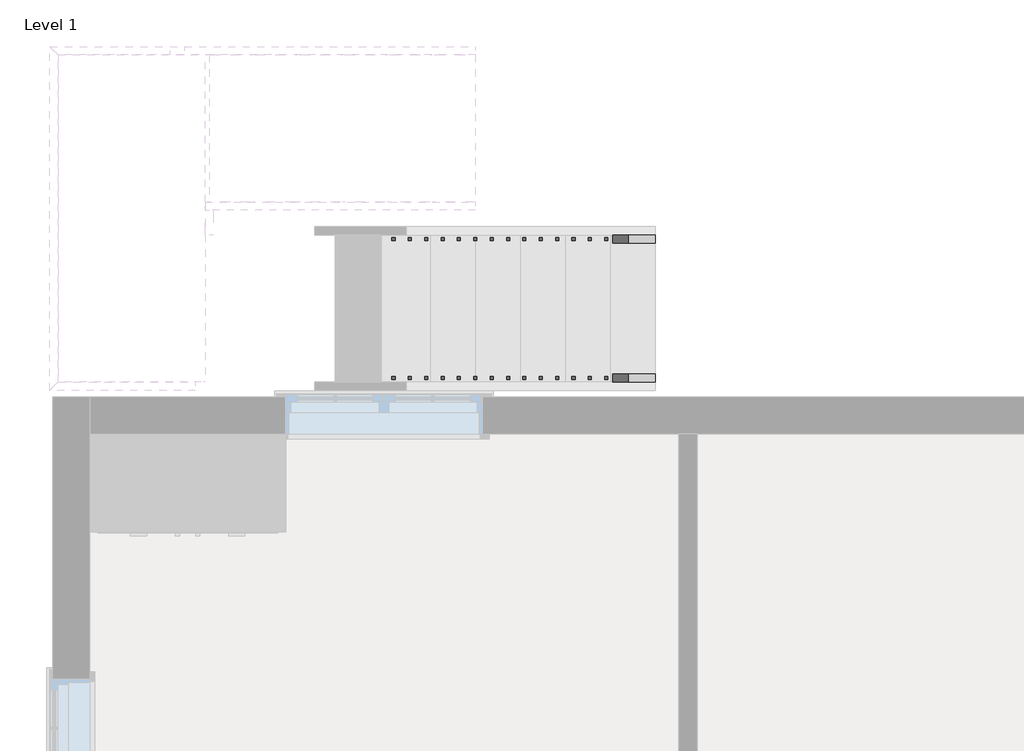
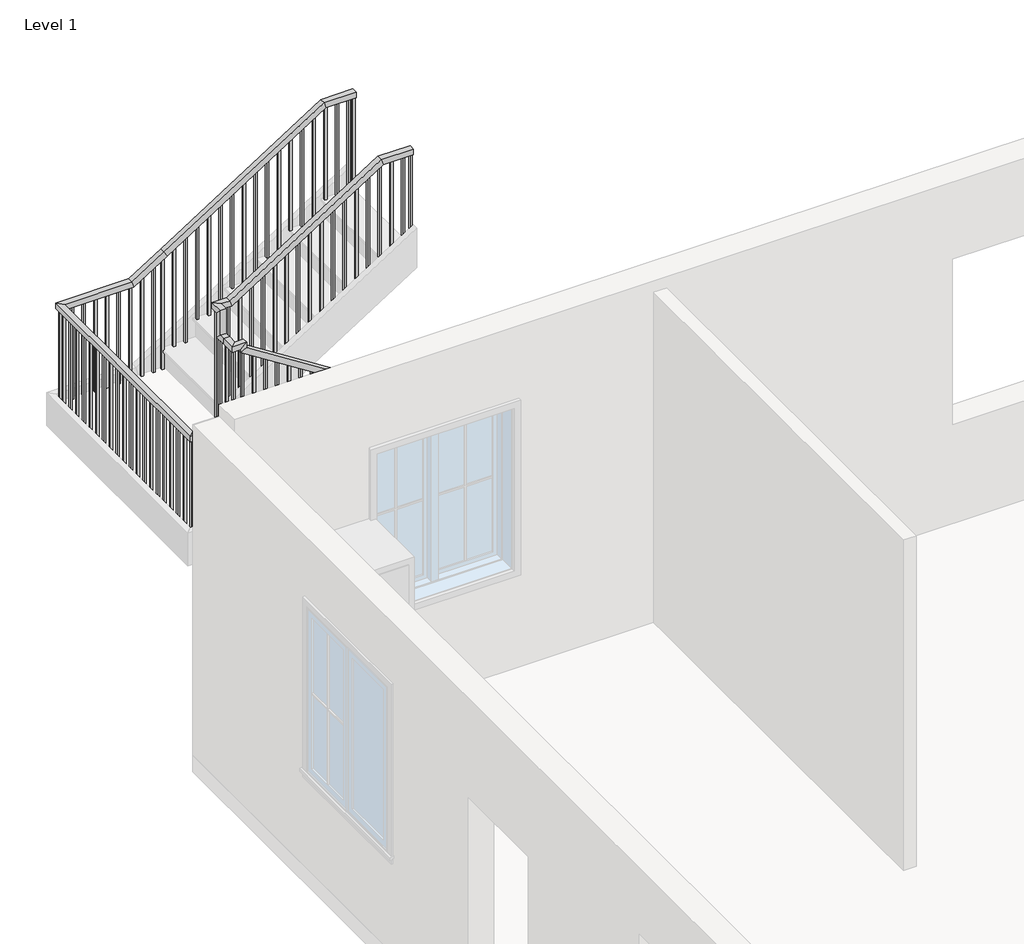
# One storey, part 2 of 3: 2 railings.
"""IFC4 building model written with IfcOpenShell, lengths in millimetres."""

from ifc_helpers import new_model, si_unit, frame, origin, place, context, project, spatial, polyline, outline, extrude, faceted_brep, element, save

model = new_model("IFC4")

# Units and contexts
model_context = context("Model", 3, world=origin())
ifc_project = project(units=[si_unit("LENGTHUNIT", "METRE", prefix="MILLI")], contexts=[model_context])

# Site, building, storey
site = spatial("IfcSite", under=ifc_project)
building = spatial("IfcBuilding", under=site)
storey = spatial("IfcBuildingStorey", under=building, Name="Level 1", Elevation=0.0)

# Railings
placement = place(None, origin())
element("IfcRailing", 1, ObjectType="Handrail - Rectangular", at=placement, inside=storey, context=model_context, shape_type="SolidModel", body=[
    faceted_brep([(13347.9752377, 21750.4384539, 1092.2), (13347.9752377, 21750.4384539, 1031.986276), (13347.9752377, 21801.2384539, 1031.986276), (13347.9752377, 21801.2384539, 1092.2), (10630.1752377, 21750.4384539, 2821.7090909), (10579.3752377, 21750.4384539, 2793.8226396), (10579.3752377, 21801.2384539, 2793.8226396), (10630.1752377, 21801.2384539, 2821.7090909), (10630.1752377, 21750.4384539, 2870.2), (10579.3752377, 21750.4384539, 2819.4), (10579.3752377, 21801.2384539, 2819.4), (10630.1752377, 21801.2384539, 2870.2), (10503.1752377, 21750.4384539, 2870.2), (10503.1752377, 21750.4384539, 2819.4), (10553.9752377, 21801.2384539, 2819.4), (10553.9752377, 21801.2384539, 2870.2), (10503.1752377, 21877.4384539, 2870.2), (10503.1752377, 21877.4384539, 2819.4), (10553.9752377, 21877.4384539, 2819.4), (10553.9752377, 21877.4384539, 2870.2), (10503.1752377, 21930.0919009, 2870.2), (10503.1752377, 21980.8919009, 2819.4), (10553.9752377, 21980.8919009, 2819.4), (10553.9752377, 21930.0919009, 2870.2), (10503.1752377, 21930.0919009, 3096.4909091), (10503.1752377, 21980.8919009, 3045.6909091), (10553.9752377, 21980.8919009, 3045.6909091), (10553.9752377, 21930.0919009, 3096.4909091), (10503.1752377, 22057.0919009, 3096.4909091), (10503.1752377, 22057.0919009, 3045.6909091), (10553.9752377, 22006.2919009, 3045.6909091), (10553.9752377, 22006.2919009, 3096.4909091), (10630.1752377, 22057.0919009, 3096.4909091), (10644.9682326, 22057.0919009, 3045.6909091), (10644.9682326, 22006.2919009, 3045.6909091), (10630.1752377, 22006.2919009, 3096.4909091), (11950.9752377, 22057.0919009, 3937.0), (11965.7682326, 22057.0919009, 3886.2), (11965.7682326, 22006.2919009, 3886.2), (11950.9752377, 22006.2919009, 3937.0), (12230.3752377, 22057.0919009, 3937.0), (12230.3752377, 22006.2919009, 3937.0), (12230.3752377, 22006.2919009, 3886.2), (12230.3752377, 22057.0919009, 3886.2)], [[[0, 1, 2, 3]], [[1, 0, 4, 5]], [[2, 1, 5, 6]], [[3, 2, 6, 7]], [[0, 3, 7, 4]], [[5, 4, 8, 9]], [[6, 5, 9, 10]], [[7, 6, 10, 11]], [[4, 7, 11, 8]], [[9, 8, 12, 13]], [[10, 9, 13, 14]], [[11, 10, 14, 15]], [[8, 11, 15, 12]], [[13, 12, 16, 17]], [[14, 13, 17, 18]], [[15, 14, 18, 19]], [[12, 15, 19, 16]], [[17, 16, 20, 21]], [[18, 17, 21, 22]], [[19, 18, 22, 23]], [[16, 19, 23, 20]], [[21, 20, 24, 25]], [[22, 21, 25, 26]], [[23, 22, 26, 27]], [[20, 23, 27, 24]], [[25, 24, 28, 29]], [[26, 25, 29, 30]], [[27, 26, 30, 31]], [[24, 27, 31, 28]], [[29, 28, 32, 33]], [[30, 29, 33, 34]], [[31, 30, 34, 35]], [[28, 31, 35, 32]], [[33, 32, 36, 37]], [[34, 33, 37, 38]], [[35, 34, 38, 39]], [[32, 35, 39, 36]], [[40, 41, 42, 43]], [[37, 36, 40, 43]], [[38, 37, 43, 42]], [[39, 38, 42, 41]], [[36, 39, 41, 40]]]),
    extrude(outline(polyline([(12144.6502377, 22022.1669009), (12144.6502377, 22041.2169009), (12163.7002377, 22041.2169009), (12163.7002377, 22022.1669009), (12144.6502377, 22022.1669009)])), frame((0.0, 0.0, 3022.6), z_axis=(0.0, 0.0, 1.0), x_axis=(1.0, 0.0, 0.0)), (0.0, 0.0, 1.0), 863.6),
    extrude(outline(polyline([(12043.0502377, 22022.1669009), (12043.0502377, 22041.2169009), (12062.1002377, 22041.2169009), (12062.1002377, 22022.1669009), (12043.0502377, 22022.1669009)])), frame((0.0, 0.0, 3022.6), z_axis=(0.0, 0.0, 1.0), x_axis=(1.0, 0.0, 0.0)), (0.0, 0.0, 1.0), 863.6),
    extrude(outline(polyline([(3882.8476396, 11960.5002377), (3870.7249123, 11941.4502377), (3022.6, 11941.4502377), (3022.6, 11960.5002377), (3882.8476396, 11960.5002377)])), frame((0.0, 22022.1669009, 0.0), z_axis=(0.0, 1.0, 0.0), x_axis=(0.0, 0.0, 1.0)), (0.0, 0.0, 1.0), 19.05),
    extrude(outline(polyline([(3818.1930941, 11858.9002377), (3806.0703669, 11839.8502377), (2844.8, 11839.8502377), (2844.8, 11858.9002377), (3818.1930941, 11858.9002377)])), frame((0.0, 22022.1669009, 0.0), z_axis=(0.0, 1.0, 0.0), x_axis=(0.0, 0.0, 1.0)), (0.0, 0.0, 1.0), 19.05),
    extrude(outline(polyline([(3753.5385487, 11757.3002377), (3741.4158214, 11738.2502377), (2844.8, 11738.2502377), (2844.8, 11757.3002377), (3753.5385487, 11757.3002377)])), frame((0.0, 22022.1669009, 0.0), z_axis=(0.0, 1.0, 0.0), x_axis=(0.0, 0.0, 1.0)), (0.0, 0.0, 1.0), 19.05),
    extrude(outline(polyline([(3688.8840032, 11655.7002377), (3676.761276, 11636.6502377), (2667.0, 11636.6502377), (2667.0, 11655.7002377), (3688.8840032, 11655.7002377)])), frame((0.0, 22022.1669009, 0.0), z_axis=(0.0, 1.0, 0.0), x_axis=(0.0, 0.0, 1.0)), (0.0, 0.0, 1.0), 19.05),
    extrude(outline(polyline([(3624.2294578, 11554.1002377), (3612.1067305, 11535.0502377), (2667.0, 11535.0502377), (2667.0, 11554.1002377), (3624.2294578, 11554.1002377)])), frame((0.0, 22022.1669009, 0.0), z_axis=(0.0, 1.0, 0.0), x_axis=(0.0, 0.0, 1.0)), (0.0, 0.0, 1.0), 19.05),
    extrude(outline(polyline([(3559.5749123, 11452.5002377), (3547.4521851, 11433.4502377), (2667.0, 11433.4502377), (2667.0, 11452.5002377), (3559.5749123, 11452.5002377)])), frame((0.0, 22022.1669009, 0.0), z_axis=(0.0, 1.0, 0.0), x_axis=(0.0, 0.0, 1.0)), (0.0, 0.0, 1.0), 19.05),
    extrude(outline(polyline([(3494.9203669, 11350.9002377), (3482.7976396, 11331.8502377), (2489.2, 11331.8502377), (2489.2, 11350.9002377), (3494.9203669, 11350.9002377)])), frame((0.0, 22022.1669009, 0.0), z_axis=(0.0, 1.0, 0.0), x_axis=(0.0, 0.0, 1.0)), (0.0, 0.0, 1.0), 19.05),
    extrude(outline(polyline([(3430.2658214, 11249.3002377), (3418.1430941, 11230.2502377), (2489.2, 11230.2502377), (2489.2, 11249.3002377), (3430.2658214, 11249.3002377)])), frame((0.0, 22022.1669009, 0.0), z_axis=(0.0, 1.0, 0.0), x_axis=(0.0, 0.0, 1.0)), (0.0, 0.0, 1.0), 19.05),
    extrude(outline(polyline([(3365.611276, 11147.7002377), (3353.4885487, 11128.6502377), (2489.2, 11128.6502377), (2489.2, 11147.7002377), (3365.611276, 11147.7002377)])), frame((0.0, 22022.1669009, 0.0), z_axis=(0.0, 1.0, 0.0), x_axis=(0.0, 0.0, 1.0)), (0.0, 0.0, 1.0), 19.05),
    extrude(outline(polyline([(3300.9567305, 11046.1002377), (3288.8340032, 11027.0502377), (2311.4, 11027.0502377), (2311.4, 11046.1002377), (3300.9567305, 11046.1002377)])), frame((0.0, 22022.1669009, 0.0), z_axis=(0.0, 1.0, 0.0), x_axis=(0.0, 0.0, 1.0)), (0.0, 0.0, 1.0), 19.05),
    extrude(outline(polyline([(3236.3021851, 10944.5002377), (3224.1794578, 10925.4502377), (2311.4, 10925.4502377), (2311.4, 10944.5002377), (3236.3021851, 10944.5002377)])), frame((0.0, 22022.1669009, 0.0), z_axis=(0.0, 1.0, 0.0), x_axis=(0.0, 0.0, 1.0)), (0.0, 0.0, 1.0), 19.05),
    extrude(outline(polyline([(3171.6476396, 10842.9002377), (3159.5249123, 10823.8502377), (2311.4, 10823.8502377), (2311.4, 10842.9002377), (3171.6476396, 10842.9002377)])), frame((0.0, 22022.1669009, 0.0), z_axis=(0.0, 1.0, 0.0), x_axis=(0.0, 0.0, 1.0)), (0.0, 0.0, 1.0), 19.05),
    extrude(outline(polyline([(3106.9930941, 10741.3002377), (3094.8703669, 10722.2502377), (2133.6, 10722.2502377), (2133.6, 10741.3002377), (3106.9930941, 10741.3002377)])), frame((0.0, 22022.1669009, 0.0), z_axis=(0.0, 1.0, 0.0), x_axis=(0.0, 0.0, 1.0)), (0.0, 0.0, 1.0), 19.05),
    extrude(outline(polyline([(3042.3385487, 10639.7002377), (3030.2158214, 10620.6502377), (2133.6, 10620.6502377), (2133.6, 10639.7002377), (3042.3385487, 10639.7002377)])), frame((0.0, 22022.1669009, 0.0), z_axis=(0.0, 1.0, 0.0), x_axis=(0.0, 0.0, 1.0)), (0.0, 0.0, 1.0), 19.05),
    extrude(outline(polyline([(10538.1002377, 21969.5134539), (10519.0502377, 21969.5134539), (10519.0502377, 21988.5634539), (10538.1002377, 21988.5634539), (10538.1002377, 21969.5134539)])), frame((0.0, 0.0, 1955.8), z_axis=(0.0, 0.0, 1.0), x_axis=(1.0, 0.0, 0.0)), (0.0, 0.0, 1.0), 1089.8909091),
    extrude(outline(polyline([(10538.1002377, 21867.9134539), (10519.0502377, 21867.9134539), (10519.0502377, 21886.9634539), (10538.1002377, 21886.9634539), (10538.1002377, 21867.9134539)])), frame((0.0, 0.0, 1955.8), z_axis=(0.0, 0.0, 1.0), x_axis=(1.0, 0.0, 0.0)), (0.0, 0.0, 1.0), 863.6),
    extrude(outline(polyline([(10614.3002377, 21785.3634539), (10614.3002377, 21766.3134539), (10595.2502377, 21766.3134539), (10595.2502377, 21785.3634539), (10614.3002377, 21785.3634539)])), frame((0.0, 0.0, 1778.0), z_axis=(0.0, 0.0, 1.0), x_axis=(1.0, 0.0, 0.0)), (0.0, 0.0, 1.0), 1041.4),
    extrude(outline(polyline([(2706.9430941, 10715.9002377), (2719.0658214, 10696.8502377), (1778.0, 10696.8502377), (1778.0, 10715.9002377), (2706.9430941, 10715.9002377)])), frame((0.0, 21766.3134539, 0.0), z_axis=(0.0, 1.0, 0.0), x_axis=(0.0, 0.0, 1.0)), (0.0, 0.0, 1.0), 19.05),
    extrude(outline(polyline([(2642.2885487, 10817.5002377), (2654.411276, 10798.4502377), (1778.0, 10798.4502377), (1778.0, 10817.5002377), (2642.2885487, 10817.5002377)])), frame((0.0, 21766.3134539, 0.0), z_axis=(0.0, 1.0, 0.0), x_axis=(0.0, 0.0, 1.0)), (0.0, 0.0, 1.0), 19.05),
    extrude(outline(polyline([(2577.6340032, 10919.1002377), (2589.7567305, 10900.0502377), (1600.2, 10900.0502377), (1600.2, 10919.1002377), (2577.6340032, 10919.1002377)])), frame((0.0, 21766.3134539, 0.0), z_axis=(0.0, 1.0, 0.0), x_axis=(0.0, 0.0, 1.0)), (0.0, 0.0, 1.0), 19.05),
    extrude(outline(polyline([(2512.9794578, 11020.7002377), (2525.1021851, 11001.6502377), (1600.2, 11001.6502377), (1600.2, 11020.7002377), (2512.9794578, 11020.7002377)])), frame((0.0, 21766.3134539, 0.0), z_axis=(0.0, 1.0, 0.0), x_axis=(0.0, 0.0, 1.0)), (0.0, 0.0, 1.0), 19.05),
    extrude(outline(polyline([(2448.3249123, 11122.3002377), (2460.4476396, 11103.2502377), (1600.2, 11103.2502377), (1600.2, 11122.3002377), (2448.3249123, 11122.3002377)])), frame((0.0, 21766.3134539, 0.0), z_axis=(0.0, 1.0, 0.0), x_axis=(0.0, 0.0, 1.0)), (0.0, 0.0, 1.0), 19.05),
    extrude(outline(polyline([(2383.6703669, 11223.9002377), (2395.7930941, 11204.8502377), (1422.4, 11204.8502377), (1422.4, 11223.9002377), (2383.6703669, 11223.9002377)])), frame((0.0, 21766.3134539, 0.0), z_axis=(0.0, 1.0, 0.0), x_axis=(0.0, 0.0, 1.0)), (0.0, 0.0, 1.0), 19.05),
    extrude(outline(polyline([(2319.0158214, 11325.5002377), (2331.1385487, 11306.4502377), (1422.4, 11306.4502377), (1422.4, 11325.5002377), (2319.0158214, 11325.5002377)])), frame((0.0, 21766.3134539, 0.0), z_axis=(0.0, 1.0, 0.0), x_axis=(0.0, 0.0, 1.0)), (0.0, 0.0, 1.0), 19.05),
    extrude(outline(polyline([(2254.361276, 11427.1002377), (2266.4840032, 11408.0502377), (1244.6, 11408.0502377), (1244.6, 11427.1002377), (2254.361276, 11427.1002377)])), frame((0.0, 21766.3134539, 0.0), z_axis=(0.0, 1.0, 0.0), x_axis=(0.0, 0.0, 1.0)), (0.0, 0.0, 1.0), 19.05),
    extrude(outline(polyline([(2189.7067305, 11528.7002377), (2201.8294578, 11509.6502377), (1244.6, 11509.6502377), (1244.6, 11528.7002377), (2189.7067305, 11528.7002377)])), frame((0.0, 21766.3134539, 0.0), z_axis=(0.0, 1.0, 0.0), x_axis=(0.0, 0.0, 1.0)), (0.0, 0.0, 1.0), 19.05),
    extrude(outline(polyline([(2125.0521851, 11630.3002377), (2137.1749123, 11611.2502377), (1244.6, 11611.2502377), (1244.6, 11630.3002377), (2125.0521851, 11630.3002377)])), frame((0.0, 21766.3134539, 0.0), z_axis=(0.0, 1.0, 0.0), x_axis=(0.0, 0.0, 1.0)), (0.0, 0.0, 1.0), 19.05),
    extrude(outline(polyline([(2060.3976396, 11731.9002377), (2072.5203669, 11712.8502377), (1066.8, 11712.8502377), (1066.8, 11731.9002377), (2060.3976396, 11731.9002377)])), frame((0.0, 21766.3134539, 0.0), z_axis=(0.0, 1.0, 0.0), x_axis=(0.0, 0.0, 1.0)), (0.0, 0.0, 1.0), 19.05),
    extrude(outline(polyline([(1995.7430941, 11833.5002377), (2007.8658214, 11814.4502377), (1066.8, 11814.4502377), (1066.8, 11833.5002377), (1995.7430941, 11833.5002377)])), frame((0.0, 21766.3134539, 0.0), z_axis=(0.0, 1.0, 0.0), x_axis=(0.0, 0.0, 1.0)), (0.0, 0.0, 1.0), 19.05),
    extrude(outline(polyline([(1931.0885487, 11935.1002377), (1943.211276, 11916.0502377), (1066.8, 11916.0502377), (1066.8, 11935.1002377), (1931.0885487, 11935.1002377)])), frame((0.0, 21766.3134539, 0.0), z_axis=(0.0, 1.0, 0.0), x_axis=(0.0, 0.0, 1.0)), (0.0, 0.0, 1.0), 19.05),
    extrude(outline(polyline([(1866.4340032, 12036.7002377), (1878.5567305, 12017.6502377), (889.0, 12017.6502377), (889.0, 12036.7002377), (1866.4340032, 12036.7002377)])), frame((0.0, 21766.3134539, 0.0), z_axis=(0.0, 1.0, 0.0), x_axis=(0.0, 0.0, 1.0)), (0.0, 0.0, 1.0), 19.05),
    extrude(outline(polyline([(1801.7794578, 12138.3002377), (1813.9021851, 12119.2502377), (889.0, 12119.2502377), (889.0, 12138.3002377), (1801.7794578, 12138.3002377)])), frame((0.0, 21766.3134539, 0.0), z_axis=(0.0, 1.0, 0.0), x_axis=(0.0, 0.0, 1.0)), (0.0, 0.0, 1.0), 19.05),
    extrude(outline(polyline([(1737.1249123, 12239.9002377), (1749.2476396, 12220.8502377), (889.0, 12220.8502377), (889.0, 12239.9002377), (1737.1249123, 12239.9002377)])), frame((0.0, 21766.3134539, 0.0), z_axis=(0.0, 1.0, 0.0), x_axis=(0.0, 0.0, 1.0)), (0.0, 0.0, 1.0), 19.05),
    extrude(outline(polyline([(1672.4703669, 12341.5002377), (1684.5930941, 12322.4502377), (711.2, 12322.4502377), (711.2, 12341.5002377), (1672.4703669, 12341.5002377)])), frame((0.0, 21766.3134539, 0.0), z_axis=(0.0, 1.0, 0.0), x_axis=(0.0, 0.0, 1.0)), (0.0, 0.0, 1.0), 19.05),
    extrude(outline(polyline([(1607.8158214, 12443.1002377), (1619.9385487, 12424.0502377), (711.2, 12424.0502377), (711.2, 12443.1002377), (1607.8158214, 12443.1002377)])), frame((0.0, 21766.3134539, 0.0), z_axis=(0.0, 1.0, 0.0), x_axis=(0.0, 0.0, 1.0)), (0.0, 0.0, 1.0), 19.05),
    extrude(outline(polyline([(1543.161276, 12544.7002377), (1555.2840032, 12525.6502377), (533.4, 12525.6502377), (533.4, 12544.7002377), (1543.161276, 12544.7002377)])), frame((0.0, 21766.3134539, 0.0), z_axis=(0.0, 1.0, 0.0), x_axis=(0.0, 0.0, 1.0)), (0.0, 0.0, 1.0), 19.05),
    extrude(outline(polyline([(1478.5067305, 12646.3002377), (1490.6294578, 12627.2502377), (533.4, 12627.2502377), (533.4, 12646.3002377), (1478.5067305, 12646.3002377)])), frame((0.0, 21766.3134539, 0.0), z_axis=(0.0, 1.0, 0.0), x_axis=(0.0, 0.0, 1.0)), (0.0, 0.0, 1.0), 19.05),
    extrude(outline(polyline([(1413.8521851, 12747.9002377), (1425.9749123, 12728.8502377), (533.4, 12728.8502377), (533.4, 12747.9002377), (1413.8521851, 12747.9002377)])), frame((0.0, 21766.3134539, 0.0), z_axis=(0.0, 1.0, 0.0), x_axis=(0.0, 0.0, 1.0)), (0.0, 0.0, 1.0), 19.05),
    extrude(outline(polyline([(1349.1976396, 12849.5002377), (1361.3203669, 12830.4502377), (355.6, 12830.4502377), (355.6, 12849.5002377), (1349.1976396, 12849.5002377)])), frame((0.0, 21766.3134539, 0.0), z_axis=(0.0, 1.0, 0.0), x_axis=(0.0, 0.0, 1.0)), (0.0, 0.0, 1.0), 19.05),
    extrude(outline(polyline([(1284.5430941, 12951.1002377), (1296.6658214, 12932.0502377), (355.6, 12932.0502377), (355.6, 12951.1002377), (1284.5430941, 12951.1002377)])), frame((0.0, 21766.3134539, 0.0), z_axis=(0.0, 1.0, 0.0), x_axis=(0.0, 0.0, 1.0)), (0.0, 0.0, 1.0), 19.05),
    extrude(outline(polyline([(1219.8885487, 13052.7002377), (1232.011276, 13033.6502377), (355.6, 13033.6502377), (355.6, 13052.7002377), (1219.8885487, 13052.7002377)])), frame((0.0, 21766.3134539, 0.0), z_axis=(0.0, 1.0, 0.0), x_axis=(0.0, 0.0, 1.0)), (0.0, 0.0, 1.0), 19.05),
    extrude(outline(polyline([(1155.2340032, 13154.3002377), (1167.3567305, 13135.2502377), (177.8, 13135.2502377), (177.8, 13154.3002377), (1155.2340032, 13154.3002377)])), frame((0.0, 21766.3134539, 0.0), z_axis=(0.0, 1.0, 0.0), x_axis=(0.0, 0.0, 1.0)), (0.0, 0.0, 1.0), 19.05),
    extrude(outline(polyline([(1090.5794578, 13255.9002377), (1102.7021851, 13236.8502377), (177.8, 13236.8502377), (177.8, 13255.9002377), (1090.5794578, 13255.9002377)])), frame((0.0, 21766.3134539, 0.0), z_axis=(0.0, 1.0, 0.0), x_axis=(0.0, 0.0, 1.0)), (0.0, 0.0, 1.0), 19.05),
    extrude(outline(polyline([(10538.1002377, 22022.1669009), (10519.0502377, 22022.1669009), (10519.0502377, 22041.2169009), (10538.1002377, 22041.2169009), (10538.1002377, 22022.1669009)])), frame((0.0, 0.0, 1955.8), z_axis=(0.0, 0.0, 1.0), x_axis=(1.0, 0.0, 0.0)), (0.0, 0.0, 1.0), 1089.8909091),
    extrude(outline(polyline([(10538.1002377, 21785.3634539), (10538.1002377, 21766.3134539), (10519.0502377, 21766.3134539), (10519.0502377, 21785.3634539), (10538.1002377, 21785.3634539)])), frame((0.0, 0.0, 1955.8), z_axis=(0.0, 0.0, 1.0), x_axis=(1.0, 0.0, 0.0)), (0.0, 0.0, 1.0), 863.6),
    extrude(outline(polyline([(12211.3252377, 22022.1669009), (12211.3252377, 22041.2169009), (12230.3752377, 22041.2169009), (12230.3752377, 22022.1669009), (12211.3252377, 22022.1669009)])), frame((0.0, 0.0, 3022.6), z_axis=(0.0, 0.0, 1.0), x_axis=(1.0, 0.0, 0.0)), (0.0, 0.0, 1.0), 863.6),
    extrude(outline(polyline([(1031.986276, 13347.9752377), (1044.1090032, 13328.9252377), (177.8, 13328.9252377), (177.8, 13347.9752377), (1031.986276, 13347.9752377)])), frame((0.0, 21766.3134539, 0.0), z_axis=(0.0, 1.0, 0.0), x_axis=(0.0, 0.0, 1.0)), (0.0, 0.0, 1.0), 19.05),
])
element("IfcRailing", 2, ObjectType="Handrail - Rectangular", at=placement, inside=storey, context=model_context, shape_type="SolidModel", body=[
    faceted_brep([(13347.9752377, 20886.8384539, 1092.2), (13347.9752377, 20886.8384539, 1031.986276), (13347.9752377, 20937.6384539, 1031.986276), (13347.9752377, 20937.6384539, 1092.2), (10553.9752377, 20886.8384539, 2870.2), (10539.1822428, 20886.8384539, 2819.4), (10539.1822428, 20937.6384539, 2819.4), (10553.9752377, 20937.6384539, 2870.2), (9639.5752377, 20886.8384539, 2870.2), (9639.5752377, 20886.8384539, 2819.4), (9690.3752377, 20937.6384539, 2819.4), (9690.3752377, 20937.6384539, 2870.2), (9639.5752377, 22920.6919009, 2870.2), (9639.5752377, 22920.6919009, 2819.4), (9690.3752377, 22869.8919009, 2819.4), (9690.3752377, 22869.8919009, 2870.2), (10274.5752377, 22920.6919009, 2870.2), (10289.3682326, 22920.6919009, 2819.4), (10289.3682326, 22869.8919009, 2819.4), (10274.5752377, 22869.8919009, 2870.2), (10553.9752377, 22920.6919009, 3048.0), (10581.2485127, 22920.6919009, 3005.1419964), (10581.2485127, 22869.8919009, 3005.1419964), (10553.9752377, 22869.8919009, 3048.0), (11950.9752377, 22920.6919009, 3937.0), (11965.7682326, 22920.6919009, 3886.2), (11965.7682326, 22869.8919009, 3886.2), (11950.9752377, 22869.8919009, 3937.0), (12230.3752377, 22920.6919009, 3937.0), (12230.3752377, 22869.8919009, 3937.0), (12230.3752377, 22869.8919009, 3886.2), (12230.3752377, 22920.6919009, 3886.2)], [[[0, 1, 2, 3]], [[1, 0, 4, 5]], [[2, 1, 5, 6]], [[3, 2, 6, 7]], [[0, 3, 7, 4]], [[5, 4, 8, 9]], [[6, 5, 9, 10]], [[7, 6, 10, 11]], [[4, 7, 11, 8]], [[9, 8, 12, 13]], [[10, 9, 13, 14]], [[11, 10, 14, 15]], [[8, 11, 15, 12]], [[13, 12, 16, 17]], [[14, 13, 17, 18]], [[15, 14, 18, 19]], [[12, 15, 19, 16]], [[17, 16, 20, 21]], [[18, 17, 21, 22]], [[19, 18, 22, 23]], [[16, 19, 23, 20]], [[21, 20, 24, 25]], [[22, 21, 25, 26]], [[23, 22, 26, 27]], [[20, 23, 27, 24]], [[28, 29, 30, 31]], [[25, 24, 28, 31]], [[26, 25, 31, 30]], [[27, 26, 30, 29]], [[24, 27, 29, 28]]]),
    extrude(outline(polyline([(12170.0502377, 22904.8169009), (12189.1002377, 22904.8169009), (12189.1002377, 22885.7669009), (12170.0502377, 22885.7669009), (12170.0502377, 22904.8169009)])), frame((0.0, 0.0, 3022.6), z_axis=(0.0, 0.0, 1.0), x_axis=(1.0, 0.0, 0.0)), (0.0, 0.0, 1.0), 863.6),
    extrude(outline(polyline([(12068.4502377, 22904.8169009), (12087.5002377, 22904.8169009), (12087.5002377, 22885.7669009), (12068.4502377, 22885.7669009), (12068.4502377, 22904.8169009)])), frame((0.0, 0.0, 3022.6), z_axis=(0.0, 0.0, 1.0), x_axis=(1.0, 0.0, 0.0)), (0.0, 0.0, 1.0), 863.6),
    extrude(outline(polyline([(11966.8502377, 22904.8169009), (11985.9002377, 22904.8169009), (11985.9002377, 22885.7669009), (11966.8502377, 22885.7669009), (11966.8502377, 22904.8169009)])), frame((0.0, 0.0, 3022.6), z_axis=(0.0, 0.0, 1.0), x_axis=(1.0, 0.0, 0.0)), (0.0, 0.0, 1.0), 863.6),
    extrude(outline(polyline([(3822.2340032, 11865.2502377), (2844.8, 11865.2502377), (2844.8, 11884.3002377), (3834.3567305, 11884.3002377), (3822.2340032, 11865.2502377)])), frame((0.0, 22885.7669009, 0.0), z_axis=(0.0, 1.0, 0.0), x_axis=(0.0, 0.0, 1.0)), (0.0, 0.0, 1.0), 19.05),
    extrude(outline(polyline([(3757.5794578, 11763.6502377), (2844.8, 11763.6502377), (2844.8, 11782.7002377), (3769.7021851, 11782.7002377), (3757.5794578, 11763.6502377)])), frame((0.0, 22885.7669009, 0.0), z_axis=(0.0, 1.0, 0.0), x_axis=(0.0, 0.0, 1.0)), (0.0, 0.0, 1.0), 19.05),
    extrude(outline(polyline([(3692.9249123, 11662.0502377), (2844.8, 11662.0502377), (2844.8, 11681.1002377), (3705.0476396, 11681.1002377), (3692.9249123, 11662.0502377)])), frame((0.0, 22885.7669009, 0.0), z_axis=(0.0, 1.0, 0.0), x_axis=(0.0, 0.0, 1.0)), (0.0, 0.0, 1.0), 19.05),
    extrude(outline(polyline([(3628.2703669, 11560.4502377), (2667.0, 11560.4502377), (2667.0, 11579.5002377), (3640.3930941, 11579.5002377), (3628.2703669, 11560.4502377)])), frame((0.0, 22885.7669009, 0.0), z_axis=(0.0, 1.0, 0.0), x_axis=(0.0, 0.0, 1.0)), (0.0, 0.0, 1.0), 19.05),
    extrude(outline(polyline([(3563.6158214, 11458.8502377), (2667.0, 11458.8502377), (2667.0, 11477.9002377), (3575.7385487, 11477.9002377), (3563.6158214, 11458.8502377)])), frame((0.0, 22885.7669009, 0.0), z_axis=(0.0, 1.0, 0.0), x_axis=(0.0, 0.0, 1.0)), (0.0, 0.0, 1.0), 19.05),
    extrude(outline(polyline([(3498.961276, 11357.2502377), (2489.2, 11357.2502377), (2489.2, 11376.3002377), (3511.0840032, 11376.3002377), (3498.961276, 11357.2502377)])), frame((0.0, 22885.7669009, 0.0), z_axis=(0.0, 1.0, 0.0), x_axis=(0.0, 0.0, 1.0)), (0.0, 0.0, 1.0), 19.05),
    extrude(outline(polyline([(3434.3067305, 11255.6502377), (2489.2, 11255.6502377), (2489.2, 11274.7002377), (3446.4294578, 11274.7002377), (3434.3067305, 11255.6502377)])), frame((0.0, 22885.7669009, 0.0), z_axis=(0.0, 1.0, 0.0), x_axis=(0.0, 0.0, 1.0)), (0.0, 0.0, 1.0), 19.05),
    extrude(outline(polyline([(3369.6521851, 11154.0502377), (2489.2, 11154.0502377), (2489.2, 11173.1002377), (3381.7749123, 11173.1002377), (3369.6521851, 11154.0502377)])), frame((0.0, 22885.7669009, 0.0), z_axis=(0.0, 1.0, 0.0), x_axis=(0.0, 0.0, 1.0)), (0.0, 0.0, 1.0), 19.05),
    extrude(outline(polyline([(3304.9976396, 11052.4502377), (2311.4, 11052.4502377), (2311.4, 11071.5002377), (3317.1203669, 11071.5002377), (3304.9976396, 11052.4502377)])), frame((0.0, 22885.7669009, 0.0), z_axis=(0.0, 1.0, 0.0), x_axis=(0.0, 0.0, 1.0)), (0.0, 0.0, 1.0), 19.05),
    extrude(outline(polyline([(3240.3430941, 10950.8502377), (2311.4, 10950.8502377), (2311.4, 10969.9002377), (3252.4658214, 10969.9002377), (3240.3430941, 10950.8502377)])), frame((0.0, 22885.7669009, 0.0), z_axis=(0.0, 1.0, 0.0), x_axis=(0.0, 0.0, 1.0)), (0.0, 0.0, 1.0), 19.05),
    extrude(outline(polyline([(3175.6885487, 10849.2502377), (2311.4, 10849.2502377), (2311.4, 10868.3002377), (3187.811276, 10868.3002377), (3175.6885487, 10849.2502377)])), frame((0.0, 22885.7669009, 0.0), z_axis=(0.0, 1.0, 0.0), x_axis=(0.0, 0.0, 1.0)), (0.0, 0.0, 1.0), 19.05),
    extrude(outline(polyline([(3111.0340032, 10747.6502377), (2133.6, 10747.6502377), (2133.6, 10766.7002377), (3123.1567305, 10766.7002377), (3111.0340032, 10747.6502377)])), frame((0.0, 22885.7669009, 0.0), z_axis=(0.0, 1.0, 0.0), x_axis=(0.0, 0.0, 1.0)), (0.0, 0.0, 1.0), 19.05),
    extrude(outline(polyline([(3046.3794578, 10646.0502377), (2133.6, 10646.0502377), (2133.6, 10665.1002377), (3058.5021851, 10665.1002377), (3046.3794578, 10646.0502377)])), frame((0.0, 22885.7669009, 0.0), z_axis=(0.0, 1.0, 0.0), x_axis=(0.0, 0.0, 1.0)), (0.0, 0.0, 1.0), 19.05),
    extrude(outline(polyline([(2933.2340032, 10468.2502377), (1955.8, 10468.2502377), (1955.8, 10487.3002377), (2945.3567305, 10487.3002377), (2933.2340032, 10468.2502377)])), frame((0.0, 22885.7669009, 0.0), z_axis=(0.0, 1.0, 0.0), x_axis=(0.0, 0.0, 1.0)), (0.0, 0.0, 1.0), 19.05),
    extrude(outline(polyline([(2868.5794578, 10366.6502377), (1955.8, 10366.6502377), (1955.8, 10385.7002377), (2880.7021851, 10385.7002377), (2868.5794578, 10366.6502377)])), frame((0.0, 22885.7669009, 0.0), z_axis=(0.0, 1.0, 0.0), x_axis=(0.0, 0.0, 1.0)), (0.0, 0.0, 1.0), 19.05),
    extrude(outline(polyline([(10265.0502377, 22904.8169009), (10284.1002377, 22904.8169009), (10284.1002377, 22885.7669009), (10265.0502377, 22885.7669009), (10265.0502377, 22904.8169009)])), frame((0.0, 0.0, 1955.8), z_axis=(0.0, 0.0, 1.0), x_axis=(1.0, 0.0, 0.0)), (0.0, 0.0, 1.0), 863.6),
    extrude(outline(polyline([(10163.4502377, 22904.8169009), (10182.5002377, 22904.8169009), (10182.5002377, 22885.7669009), (10163.4502377, 22885.7669009), (10163.4502377, 22904.8169009)])), frame((0.0, 0.0, 1955.8), z_axis=(0.0, 0.0, 1.0), x_axis=(1.0, 0.0, 0.0)), (0.0, 0.0, 1.0), 863.6),
    extrude(outline(polyline([(10061.8502377, 22904.8169009), (10080.9002377, 22904.8169009), (10080.9002377, 22885.7669009), (10061.8502377, 22885.7669009), (10061.8502377, 22904.8169009)])), frame((0.0, 0.0, 1955.8), z_axis=(0.0, 0.0, 1.0), x_axis=(1.0, 0.0, 0.0)), (0.0, 0.0, 1.0), 863.6),
    extrude(outline(polyline([(9960.2502377, 22904.8169009), (9979.3002377, 22904.8169009), (9979.3002377, 22885.7669009), (9960.2502377, 22885.7669009), (9960.2502377, 22904.8169009)])), frame((0.0, 0.0, 1955.8), z_axis=(0.0, 0.0, 1.0), x_axis=(1.0, 0.0, 0.0)), (0.0, 0.0, 1.0), 863.6),
    extrude(outline(polyline([(9858.6502377, 22904.8169009), (9877.7002377, 22904.8169009), (9877.7002377, 22885.7669009), (9858.6502377, 22885.7669009), (9858.6502377, 22904.8169009)])), frame((0.0, 0.0, 1955.8), z_axis=(0.0, 0.0, 1.0), x_axis=(1.0, 0.0, 0.0)), (0.0, 0.0, 1.0), 863.6),
    extrude(outline(polyline([(9757.0502377, 22904.8169009), (9776.1002377, 22904.8169009), (9776.1002377, 22885.7669009), (9757.0502377, 22885.7669009), (9757.0502377, 22904.8169009)])), frame((0.0, 0.0, 1955.8), z_axis=(0.0, 0.0, 1.0), x_axis=(1.0, 0.0, 0.0)), (0.0, 0.0, 1.0), 863.6),
    extrude(outline(polyline([(9655.4502377, 22833.1134539), (9655.4502377, 22852.1634539), (9674.5002377, 22852.1634539), (9674.5002377, 22833.1134539), (9655.4502377, 22833.1134539)])), frame((0.0, 0.0, 1955.8), z_axis=(0.0, 0.0, 1.0), x_axis=(1.0, 0.0, 0.0)), (0.0, 0.0, 1.0), 863.6),
    extrude(outline(polyline([(9655.4502377, 22731.5134539), (9655.4502377, 22750.5634539), (9674.5002377, 22750.5634539), (9674.5002377, 22731.5134539), (9655.4502377, 22731.5134539)])), frame((0.0, 0.0, 1955.8), z_axis=(0.0, 0.0, 1.0), x_axis=(1.0, 0.0, 0.0)), (0.0, 0.0, 1.0), 863.6),
    extrude(outline(polyline([(9655.4502377, 22629.9134539), (9655.4502377, 22648.9634539), (9674.5002377, 22648.9634539), (9674.5002377, 22629.9134539), (9655.4502377, 22629.9134539)])), frame((0.0, 0.0, 1955.8), z_axis=(0.0, 0.0, 1.0), x_axis=(1.0, 0.0, 0.0)), (0.0, 0.0, 1.0), 863.6),
    extrude(outline(polyline([(9655.4502377, 22528.3134539), (9655.4502377, 22547.3634539), (9674.5002377, 22547.3634539), (9674.5002377, 22528.3134539), (9655.4502377, 22528.3134539)])), frame((0.0, 0.0, 1955.8), z_axis=(0.0, 0.0, 1.0), x_axis=(1.0, 0.0, 0.0)), (0.0, 0.0, 1.0), 863.6),
    extrude(outline(polyline([(9655.4502377, 22426.7134539), (9655.4502377, 22445.7634539), (9674.5002377, 22445.7634539), (9674.5002377, 22426.7134539), (9655.4502377, 22426.7134539)])), frame((0.0, 0.0, 1955.8), z_axis=(0.0, 0.0, 1.0), x_axis=(1.0, 0.0, 0.0)), (0.0, 0.0, 1.0), 863.6),
    extrude(outline(polyline([(9655.4502377, 22325.1134539), (9655.4502377, 22344.1634539), (9674.5002377, 22344.1634539), (9674.5002377, 22325.1134539), (9655.4502377, 22325.1134539)])), frame((0.0, 0.0, 1955.8), z_axis=(0.0, 0.0, 1.0), x_axis=(1.0, 0.0, 0.0)), (0.0, 0.0, 1.0), 863.6),
    extrude(outline(polyline([(9655.4502377, 22223.5134539), (9655.4502377, 22242.5634539), (9674.5002377, 22242.5634539), (9674.5002377, 22223.5134539), (9655.4502377, 22223.5134539)])), frame((0.0, 0.0, 1955.8), z_axis=(0.0, 0.0, 1.0), x_axis=(1.0, 0.0, 0.0)), (0.0, 0.0, 1.0), 863.6),
    extrude(outline(polyline([(9655.4502377, 22121.9134539), (9655.4502377, 22140.9634539), (9674.5002377, 22140.9634539), (9674.5002377, 22121.9134539), (9655.4502377, 22121.9134539)])), frame((0.0, 0.0, 1955.8), z_axis=(0.0, 0.0, 1.0), x_axis=(1.0, 0.0, 0.0)), (0.0, 0.0, 1.0), 863.6),
    extrude(outline(polyline([(9655.4502377, 22020.3134539), (9655.4502377, 22039.3634539), (9674.5002377, 22039.3634539), (9674.5002377, 22020.3134539), (9655.4502377, 22020.3134539)])), frame((0.0, 0.0, 1955.8), z_axis=(0.0, 0.0, 1.0), x_axis=(1.0, 0.0, 0.0)), (0.0, 0.0, 1.0), 863.6),
    extrude(outline(polyline([(9655.4502377, 21918.7134539), (9655.4502377, 21937.7634539), (9674.5002377, 21937.7634539), (9674.5002377, 21918.7134539), (9655.4502377, 21918.7134539)])), frame((0.0, 0.0, 1955.8), z_axis=(0.0, 0.0, 1.0), x_axis=(1.0, 0.0, 0.0)), (0.0, 0.0, 1.0), 863.6),
    extrude(outline(polyline([(9655.4502377, 21817.1134539), (9655.4502377, 21836.1634539), (9674.5002377, 21836.1634539), (9674.5002377, 21817.1134539), (9655.4502377, 21817.1134539)])), frame((0.0, 0.0, 1955.8), z_axis=(0.0, 0.0, 1.0), x_axis=(1.0, 0.0, 0.0)), (0.0, 0.0, 1.0), 863.6),
    extrude(outline(polyline([(9655.4502377, 21715.5134539), (9655.4502377, 21734.5634539), (9674.5002377, 21734.5634539), (9674.5002377, 21715.5134539), (9655.4502377, 21715.5134539)])), frame((0.0, 0.0, 1955.8), z_axis=(0.0, 0.0, 1.0), x_axis=(1.0, 0.0, 0.0)), (0.0, 0.0, 1.0), 863.6),
    extrude(outline(polyline([(9655.4502377, 21613.9134539), (9655.4502377, 21632.9634539), (9674.5002377, 21632.9634539), (9674.5002377, 21613.9134539), (9655.4502377, 21613.9134539)])), frame((0.0, 0.0, 1955.8), z_axis=(0.0, 0.0, 1.0), x_axis=(1.0, 0.0, 0.0)), (0.0, 0.0, 1.0), 863.6),
    extrude(outline(polyline([(9655.4502377, 21512.3134539), (9655.4502377, 21531.3634539), (9674.5002377, 21531.3634539), (9674.5002377, 21512.3134539), (9655.4502377, 21512.3134539)])), frame((0.0, 0.0, 1955.8), z_axis=(0.0, 0.0, 1.0), x_axis=(1.0, 0.0, 0.0)), (0.0, 0.0, 1.0), 863.6),
    extrude(outline(polyline([(9655.4502377, 21410.7134539), (9655.4502377, 21429.7634539), (9674.5002377, 21429.7634539), (9674.5002377, 21410.7134539), (9655.4502377, 21410.7134539)])), frame((0.0, 0.0, 1955.8), z_axis=(0.0, 0.0, 1.0), x_axis=(1.0, 0.0, 0.0)), (0.0, 0.0, 1.0), 863.6),
    extrude(outline(polyline([(9655.4502377, 21309.1134539), (9655.4502377, 21328.1634539), (9674.5002377, 21328.1634539), (9674.5002377, 21309.1134539), (9655.4502377, 21309.1134539)])), frame((0.0, 0.0, 1955.8), z_axis=(0.0, 0.0, 1.0), x_axis=(1.0, 0.0, 0.0)), (0.0, 0.0, 1.0), 863.6),
    extrude(outline(polyline([(9655.4502377, 21207.5134539), (9655.4502377, 21226.5634539), (9674.5002377, 21226.5634539), (9674.5002377, 21207.5134539), (9655.4502377, 21207.5134539)])), frame((0.0, 0.0, 1955.8), z_axis=(0.0, 0.0, 1.0), x_axis=(1.0, 0.0, 0.0)), (0.0, 0.0, 1.0), 863.6),
    extrude(outline(polyline([(9655.4502377, 21105.9134539), (9655.4502377, 21124.9634539), (9674.5002377, 21124.9634539), (9674.5002377, 21105.9134539), (9655.4502377, 21105.9134539)])), frame((0.0, 0.0, 1955.8), z_axis=(0.0, 0.0, 1.0), x_axis=(1.0, 0.0, 0.0)), (0.0, 0.0, 1.0), 863.6),
    extrude(outline(polyline([(9655.4502377, 21004.3134539), (9655.4502377, 21023.3634539), (9674.5002377, 21023.3634539), (9674.5002377, 21004.3134539), (9655.4502377, 21004.3134539)])), frame((0.0, 0.0, 1955.8), z_axis=(0.0, 0.0, 1.0), x_axis=(1.0, 0.0, 0.0)), (0.0, 0.0, 1.0), 863.6),
    extrude(outline(polyline([(9750.7002377, 20902.7134539), (9731.6502377, 20902.7134539), (9731.6502377, 20921.7634539), (9750.7002377, 20921.7634539), (9750.7002377, 20902.7134539)])), frame((0.0, 0.0, 1955.8), z_axis=(0.0, 0.0, 1.0), x_axis=(1.0, 0.0, 0.0)), (0.0, 0.0, 1.0), 863.6),
    extrude(outline(polyline([(9852.3002377, 20902.7134539), (9833.2502377, 20902.7134539), (9833.2502377, 20921.7634539), (9852.3002377, 20921.7634539), (9852.3002377, 20902.7134539)])), frame((0.0, 0.0, 1955.8), z_axis=(0.0, 0.0, 1.0), x_axis=(1.0, 0.0, 0.0)), (0.0, 0.0, 1.0), 863.6),
    extrude(outline(polyline([(9953.9002377, 20902.7134539), (9934.8502377, 20902.7134539), (9934.8502377, 20921.7634539), (9953.9002377, 20921.7634539), (9953.9002377, 20902.7134539)])), frame((0.0, 0.0, 1955.8), z_axis=(0.0, 0.0, 1.0), x_axis=(1.0, 0.0, 0.0)), (0.0, 0.0, 1.0), 863.6),
    extrude(outline(polyline([(10055.5002377, 20902.7134539), (10036.4502377, 20902.7134539), (10036.4502377, 20921.7634539), (10055.5002377, 20921.7634539), (10055.5002377, 20902.7134539)])), frame((0.0, 0.0, 1955.8), z_axis=(0.0, 0.0, 1.0), x_axis=(1.0, 0.0, 0.0)), (0.0, 0.0, 1.0), 863.6),
    extrude(outline(polyline([(10157.1002377, 20902.7134539), (10138.0502377, 20902.7134539), (10138.0502377, 20921.7634539), (10157.1002377, 20921.7634539), (10157.1002377, 20902.7134539)])), frame((0.0, 0.0, 1955.8), z_axis=(0.0, 0.0, 1.0), x_axis=(1.0, 0.0, 0.0)), (0.0, 0.0, 1.0), 863.6),
    extrude(outline(polyline([(10258.7002377, 20902.7134539), (10239.6502377, 20902.7134539), (10239.6502377, 20921.7634539), (10258.7002377, 20921.7634539), (10258.7002377, 20902.7134539)])), frame((0.0, 0.0, 1955.8), z_axis=(0.0, 0.0, 1.0), x_axis=(1.0, 0.0, 0.0)), (0.0, 0.0, 1.0), 863.6),
    extrude(outline(polyline([(10360.3002377, 20902.7134539), (10341.2502377, 20902.7134539), (10341.2502377, 20921.7634539), (10360.3002377, 20921.7634539), (10360.3002377, 20902.7134539)])), frame((0.0, 0.0, 1955.8), z_axis=(0.0, 0.0, 1.0), x_axis=(1.0, 0.0, 0.0)), (0.0, 0.0, 1.0), 863.6),
    extrude(outline(polyline([(10461.9002377, 20902.7134539), (10442.8502377, 20902.7134539), (10442.8502377, 20921.7634539), (10461.9002377, 20921.7634539), (10461.9002377, 20902.7134539)])), frame((0.0, 0.0, 1955.8), z_axis=(0.0, 0.0, 1.0), x_axis=(1.0, 0.0, 0.0)), (0.0, 0.0, 1.0), 863.6),
    extrude(outline(polyline([(2783.7203669, 10595.2502377), (1778.0, 10595.2502377), (1778.0, 10614.3002377), (2771.5976396, 10614.3002377), (2783.7203669, 10595.2502377)])), frame((0.0, 20902.7134539, 0.0), z_axis=(0.0, 1.0, 0.0), x_axis=(0.0, 0.0, 1.0)), (0.0, 0.0, 1.0), 19.05),
    extrude(outline(polyline([(2719.0658214, 10696.8502377), (1778.0, 10696.8502377), (1778.0, 10715.9002377), (2706.9430941, 10715.9002377), (2719.0658214, 10696.8502377)])), frame((0.0, 20902.7134539, 0.0), z_axis=(0.0, 1.0, 0.0), x_axis=(0.0, 0.0, 1.0)), (0.0, 0.0, 1.0), 19.05),
    extrude(outline(polyline([(2654.411276, 10798.4502377), (1778.0, 10798.4502377), (1778.0, 10817.5002377), (2642.2885487, 10817.5002377), (2654.411276, 10798.4502377)])), frame((0.0, 20902.7134539, 0.0), z_axis=(0.0, 1.0, 0.0), x_axis=(0.0, 0.0, 1.0)), (0.0, 0.0, 1.0), 19.05),
    extrude(outline(polyline([(2589.7567305, 10900.0502377), (1600.2, 10900.0502377), (1600.2, 10919.1002377), (2577.6340032, 10919.1002377), (2589.7567305, 10900.0502377)])), frame((0.0, 20902.7134539, 0.0), z_axis=(0.0, 1.0, 0.0), x_axis=(0.0, 0.0, 1.0)), (0.0, 0.0, 1.0), 19.05),
    extrude(outline(polyline([(2525.1021851, 11001.6502377), (1600.2, 11001.6502377), (1600.2, 11020.7002377), (2512.9794578, 11020.7002377), (2525.1021851, 11001.6502377)])), frame((0.0, 20902.7134539, 0.0), z_axis=(0.0, 1.0, 0.0), x_axis=(0.0, 0.0, 1.0)), (0.0, 0.0, 1.0), 19.05),
    extrude(outline(polyline([(2460.4476396, 11103.2502377), (1600.2, 11103.2502377), (1600.2, 11122.3002377), (2448.3249123, 11122.3002377), (2460.4476396, 11103.2502377)])), frame((0.0, 20902.7134539, 0.0), z_axis=(0.0, 1.0, 0.0), x_axis=(0.0, 0.0, 1.0)), (0.0, 0.0, 1.0), 19.05),
    extrude(outline(polyline([(2395.7930941, 11204.8502377), (1422.4, 11204.8502377), (1422.4, 11223.9002377), (2383.6703669, 11223.9002377), (2395.7930941, 11204.8502377)])), frame((0.0, 20902.7134539, 0.0), z_axis=(0.0, 1.0, 0.0), x_axis=(0.0, 0.0, 1.0)), (0.0, 0.0, 1.0), 19.05),
    extrude(outline(polyline([(2331.1385487, 11306.4502377), (1422.4, 11306.4502377), (1422.4, 11325.5002377), (2319.0158214, 11325.5002377), (2331.1385487, 11306.4502377)])), frame((0.0, 20902.7134539, 0.0), z_axis=(0.0, 1.0, 0.0), x_axis=(0.0, 0.0, 1.0)), (0.0, 0.0, 1.0), 19.05),
    extrude(outline(polyline([(2266.4840032, 11408.0502377), (1244.6, 11408.0502377), (1244.6, 11427.1002377), (2254.361276, 11427.1002377), (2266.4840032, 11408.0502377)])), frame((0.0, 20902.7134539, 0.0), z_axis=(0.0, 1.0, 0.0), x_axis=(0.0, 0.0, 1.0)), (0.0, 0.0, 1.0), 19.05),
    extrude(outline(polyline([(2201.8294578, 11509.6502377), (1244.6, 11509.6502377), (1244.6, 11528.7002377), (2189.7067305, 11528.7002377), (2201.8294578, 11509.6502377)])), frame((0.0, 20902.7134539, 0.0), z_axis=(0.0, 1.0, 0.0), x_axis=(0.0, 0.0, 1.0)), (0.0, 0.0, 1.0), 19.05),
    extrude(outline(polyline([(2137.1749123, 11611.2502377), (1244.6, 11611.2502377), (1244.6, 11630.3002377), (2125.0521851, 11630.3002377), (2137.1749123, 11611.2502377)])), frame((0.0, 20902.7134539, 0.0), z_axis=(0.0, 1.0, 0.0), x_axis=(0.0, 0.0, 1.0)), (0.0, 0.0, 1.0), 19.05),
    extrude(outline(polyline([(2072.5203669, 11712.8502377), (1066.8, 11712.8502377), (1066.8, 11731.9002377), (2060.3976396, 11731.9002377), (2072.5203669, 11712.8502377)])), frame((0.0, 20902.7134539, 0.0), z_axis=(0.0, 1.0, 0.0), x_axis=(0.0, 0.0, 1.0)), (0.0, 0.0, 1.0), 19.05),
    extrude(outline(polyline([(2007.8658214, 11814.4502377), (1066.8, 11814.4502377), (1066.8, 11833.5002377), (1995.7430941, 11833.5002377), (2007.8658214, 11814.4502377)])), frame((0.0, 20902.7134539, 0.0), z_axis=(0.0, 1.0, 0.0), x_axis=(0.0, 0.0, 1.0)), (0.0, 0.0, 1.0), 19.05),
    extrude(outline(polyline([(1943.211276, 11916.0502377), (1066.8, 11916.0502377), (1066.8, 11935.1002377), (1931.0885487, 11935.1002377), (1943.211276, 11916.0502377)])), frame((0.0, 20902.7134539, 0.0), z_axis=(0.0, 1.0, 0.0), x_axis=(0.0, 0.0, 1.0)), (0.0, 0.0, 1.0), 19.05),
    extrude(outline(polyline([(1878.5567305, 12017.6502377), (889.0, 12017.6502377), (889.0, 12036.7002377), (1866.4340032, 12036.7002377), (1878.5567305, 12017.6502377)])), frame((0.0, 20902.7134539, 0.0), z_axis=(0.0, 1.0, 0.0), x_axis=(0.0, 0.0, 1.0)), (0.0, 0.0, 1.0), 19.05),
    extrude(outline(polyline([(1813.9021851, 12119.2502377), (889.0, 12119.2502377), (889.0, 12138.3002377), (1801.7794578, 12138.3002377), (1813.9021851, 12119.2502377)])), frame((0.0, 20902.7134539, 0.0), z_axis=(0.0, 1.0, 0.0), x_axis=(0.0, 0.0, 1.0)), (0.0, 0.0, 1.0), 19.05),
    extrude(outline(polyline([(1749.2476396, 12220.8502377), (889.0, 12220.8502377), (889.0, 12239.9002377), (1737.1249123, 12239.9002377), (1749.2476396, 12220.8502377)])), frame((0.0, 20902.7134539, 0.0), z_axis=(0.0, 1.0, 0.0), x_axis=(0.0, 0.0, 1.0)), (0.0, 0.0, 1.0), 19.05),
    extrude(outline(polyline([(1684.5930941, 12322.4502377), (711.2, 12322.4502377), (711.2, 12341.5002377), (1672.4703669, 12341.5002377), (1684.5930941, 12322.4502377)])), frame((0.0, 20902.7134539, 0.0), z_axis=(0.0, 1.0, 0.0), x_axis=(0.0, 0.0, 1.0)), (0.0, 0.0, 1.0), 19.05),
    extrude(outline(polyline([(1619.9385487, 12424.0502377), (711.2, 12424.0502377), (711.2, 12443.1002377), (1607.8158214, 12443.1002377), (1619.9385487, 12424.0502377)])), frame((0.0, 20902.7134539, 0.0), z_axis=(0.0, 1.0, 0.0), x_axis=(0.0, 0.0, 1.0)), (0.0, 0.0, 1.0), 19.05),
    extrude(outline(polyline([(1555.2840032, 12525.6502377), (533.4, 12525.6502377), (533.4, 12544.7002377), (1543.161276, 12544.7002377), (1555.2840032, 12525.6502377)])), frame((0.0, 20902.7134539, 0.0), z_axis=(0.0, 1.0, 0.0), x_axis=(0.0, 0.0, 1.0)), (0.0, 0.0, 1.0), 19.05),
    extrude(outline(polyline([(1490.6294578, 12627.2502377), (533.4, 12627.2502377), (533.4, 12646.3002377), (1478.5067305, 12646.3002377), (1490.6294578, 12627.2502377)])), frame((0.0, 20902.7134539, 0.0), z_axis=(0.0, 1.0, 0.0), x_axis=(0.0, 0.0, 1.0)), (0.0, 0.0, 1.0), 19.05),
    extrude(outline(polyline([(1425.9749123, 12728.8502377), (533.4, 12728.8502377), (533.4, 12747.9002377), (1413.8521851, 12747.9002377), (1425.9749123, 12728.8502377)])), frame((0.0, 20902.7134539, 0.0), z_axis=(0.0, 1.0, 0.0), x_axis=(0.0, 0.0, 1.0)), (0.0, 0.0, 1.0), 19.05),
    extrude(outline(polyline([(1361.3203669, 12830.4502377), (355.6, 12830.4502377), (355.6, 12849.5002377), (1349.1976396, 12849.5002377), (1361.3203669, 12830.4502377)])), frame((0.0, 20902.7134539, 0.0), z_axis=(0.0, 1.0, 0.0), x_axis=(0.0, 0.0, 1.0)), (0.0, 0.0, 1.0), 19.05),
    extrude(outline(polyline([(1296.6658214, 12932.0502377), (355.6, 12932.0502377), (355.6, 12951.1002377), (1284.5430941, 12951.1002377), (1296.6658214, 12932.0502377)])), frame((0.0, 20902.7134539, 0.0), z_axis=(0.0, 1.0, 0.0), x_axis=(0.0, 0.0, 1.0)), (0.0, 0.0, 1.0), 19.05),
    extrude(outline(polyline([(1232.011276, 13033.6502377), (355.6, 13033.6502377), (355.6, 13052.7002377), (1219.8885487, 13052.7002377), (1232.011276, 13033.6502377)])), frame((0.0, 20902.7134539, 0.0), z_axis=(0.0, 1.0, 0.0), x_axis=(0.0, 0.0, 1.0)), (0.0, 0.0, 1.0), 19.05),
    extrude(outline(polyline([(1167.3567305, 13135.2502377), (177.8, 13135.2502377), (177.8, 13154.3002377), (1155.2340032, 13154.3002377), (1167.3567305, 13135.2502377)])), frame((0.0, 20902.7134539, 0.0), z_axis=(0.0, 1.0, 0.0), x_axis=(0.0, 0.0, 1.0)), (0.0, 0.0, 1.0), 19.05),
    extrude(outline(polyline([(1102.7021851, 13236.8502377), (177.8, 13236.8502377), (177.8, 13255.9002377), (1090.5794578, 13255.9002377), (1102.7021851, 13236.8502377)])), frame((0.0, 20902.7134539, 0.0), z_axis=(0.0, 1.0, 0.0), x_axis=(0.0, 0.0, 1.0)), (0.0, 0.0, 1.0), 19.05),
    extrude(outline(polyline([(2981.7249123, 10544.4502377), (1955.8, 10544.4502377), (1955.8, 10563.5002377), (2993.8476396, 10563.5002377), (2981.7249123, 10544.4502377)])), frame((0.0, 22885.7669009, 0.0), z_axis=(0.0, 1.0, 0.0), x_axis=(0.0, 0.0, 1.0)), (0.0, 0.0, 1.0), 19.05),
    extrude(outline(polyline([(9655.4502377, 22885.7669009), (9655.4502377, 22904.8169009), (9674.5002377, 22904.8169009), (9674.5002377, 22885.7669009), (9655.4502377, 22885.7669009)])), frame((0.0, 0.0, 1955.8), z_axis=(0.0, 0.0, 1.0), x_axis=(1.0, 0.0, 0.0)), (0.0, 0.0, 1.0), 863.6),
    extrude(outline(polyline([(9674.5002377, 20902.7134539), (9655.4502377, 20902.7134539), (9655.4502377, 20921.7634539), (9674.5002377, 20921.7634539), (9674.5002377, 20902.7134539)])), frame((0.0, 0.0, 1955.8), z_axis=(0.0, 0.0, 1.0), x_axis=(1.0, 0.0, 0.0)), (0.0, 0.0, 1.0), 863.6),
    extrude(outline(polyline([(2816.0476396, 10544.4502377), (1955.8, 10544.4502377), (1955.8, 10563.5002377), (2803.9249123, 10563.5002377), (2816.0476396, 10544.4502377)])), frame((0.0, 20902.7134539, 0.0), z_axis=(0.0, 1.0, 0.0), x_axis=(0.0, 0.0, 1.0)), (0.0, 0.0, 1.0), 19.05),
    extrude(outline(polyline([(12211.3252377, 22904.8169009), (12230.3752377, 22904.8169009), (12230.3752377, 22885.7669009), (12211.3252377, 22885.7669009), (12211.3252377, 22904.8169009)])), frame((0.0, 0.0, 3022.6), z_axis=(0.0, 0.0, 1.0), x_axis=(1.0, 0.0, 0.0)), (0.0, 0.0, 1.0), 863.6),
    extrude(outline(polyline([(1044.1090032, 13328.9252377), (177.8, 13328.9252377), (177.8, 13347.9752377), (1031.986276, 13347.9752377), (1044.1090032, 13328.9252377)])), frame((0.0, 20902.7134539, 0.0), z_axis=(0.0, 1.0, 0.0), x_axis=(0.0, 0.0, 1.0)), (0.0, 0.0, 1.0), 19.05),
])

save(model, "model.ifc")

# Revit data of these elements
# Type "Handrail - Rectangular"
#   Assembly Code = "C2010400"
#   built-in parameter 1008612 = 0.0416667 (stored number, unit not read)
#   built-in parameter 1008611 = 0.0416667 (stored number, unit not read)
#   built-in parameter 1008609 = 0.333333 (stored number, unit not read)
#   built-in parameter 1008604 = 0.166667 (stored number, unit not read)
#   built-in parameter 1008603 = 0.166667 (stored number, unit not read)
#   Railing Height = 3' - 0"
#   built-in parameter 1008630 = 2
#   built-in parameter 1008610 = 2
#   built-in parameter 1008618 = Baluster - Square : 3/4"
# Elements 1, 2 (IfcRailing, "Handrail - Rectangular")
#   Phase Created = New Construction
